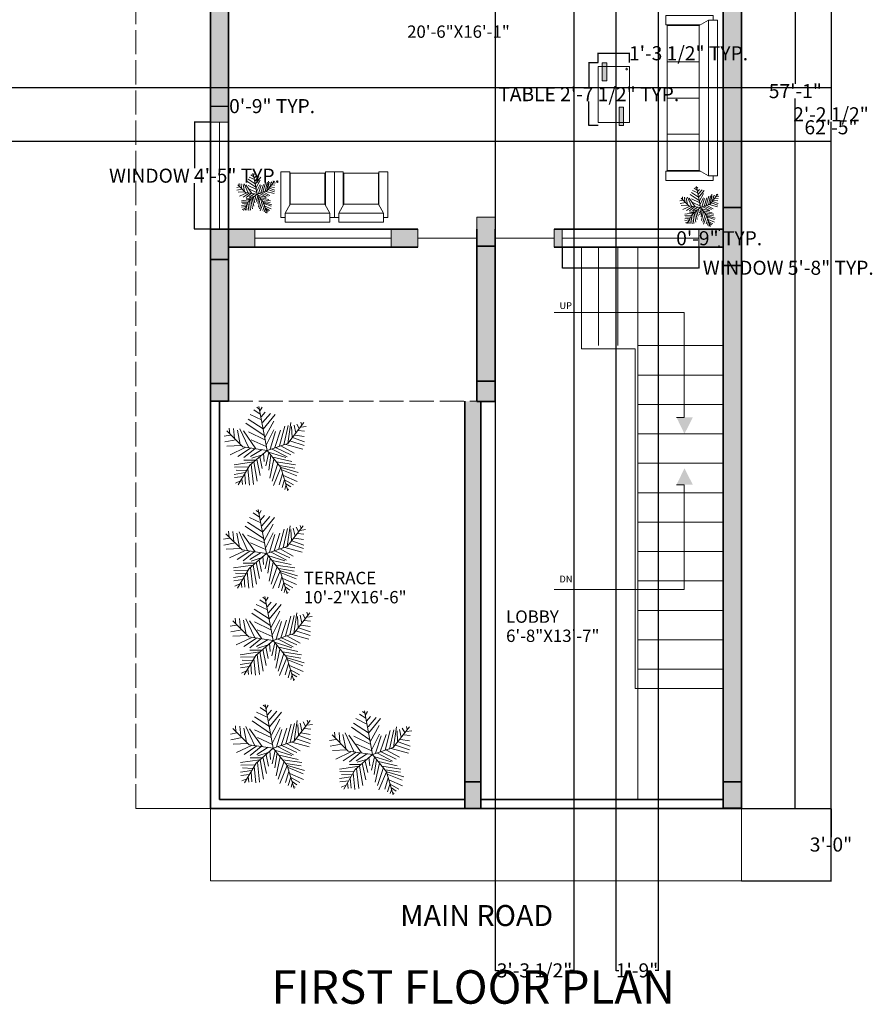
# Model space of a CAD drawing. Units: inches. Extents: x -17 to 892, y -721 to 172.
# Tile 7 of 11: x 438 to 862, y -721 to -231. Entities that reach past the tile are written whole.
import ezdxf

# ---------------------------------------------------------------- set-up
doc = ezdxf.new("R2010")
doc.units = ezdxf.units.IN
doc.header["$MEASUREMENT"] = 0
doc.linetypes.add('ACAD_ISO02W100', pattern=[15, 12, -3])
doc.layers.get('0').update_dxf_attribs({"color": 14})
for name, color, linetype, lineweight in [('A-ANNO-DIMS', 2, 'Continuous', 18), ('A-ANNO-SYMB', 7, 'Continuous', 18), ('A-ANNO-TEXT', 7, 'Continuous', 18), ('A-ANNO-TITL', 7, 'Continuous', 35), ('A-AREA-IDEN', 7, 'Continuous', 18), ('A-COLS', 252, 'Continuous', 35), ('A-FLOR-OVHD', 252, 'ACAD_ISO02W100', 18), ('A-FLOR-STRS', 8, 'Continuous', 18), ('A-WALL-PATT', 14, 'Continuous', 13), ('C-PROP', 8, 'ACAD_ISO02W100', 18), ('C-ROAD', 8, 'Continuous', 18), ('doors', 4, 'Continuous', 18), ('furniture', 252, 'Continuous', 18), ('lawn', 102, 'Continuous', 13), ('walls', 252, 'Continuous', 35), ('windows', 161, 'Continuous', 18)]:
    doc.layers.add(name, color=color, linetype=linetype, lineweight=lineweight)
doc.layers.add('A-COLS-PATT', color=254, linetype='Continuous', lineweight=13, true_color=0xd7ebd2)
doc.styles.get("Standard").update_dxf_attribs({"font": 'arial.ttf'})
doc.dimstyles.get("Standard").update_dxf_attribs({"dimtxt": 7, "dimasz": 0.18, "dimexe": 0.18, "dimexo": 0.0625, "dimgap": 0.09, "dimtad": 0, "dimtih": 1, "dimtoh": 1, "dimzin": 0, "dimdsep": 46, "dimlunit": 3, "dimtxsty": 'Standard', "dimcen": 0.09, "dimadec": 0, "dimazin": 0, "dimtfac": 1, "dimtofl": 0, "dimtmove": 0, "dimatfit": 3, "dimfxl": 1, "dimtolj": 1, "dimtzin": 0, "dimarcsym": 0})

# ---------------------------------------------------------------- blocks, each defined once
blk = doc.blocks.new('FABRIC SOFA 4S')
at = {"layer": 'furniture'}
for p, q in [((3, 54), (34, 54)), ((3, 51), (3, 54)), ((34, 48), (34, 54)), ((0, -51), (0, 51)), ((6, 51), (0, 51)), ((6, -51), (6, 51)), ((12, 47.63), (6, 51)), ((11.14, 48), (34, 48)), ((33, 23.81), (12, 23.81)), ((33, 0), (12, 0)), ((33, -23.81), (12, -23.81)), ((6, -51), (0, -51)), ((3, -54), (3, -51)), ((6, -51), (12, -47.63)), ((11.54, -48), (34, -48)), ((34, -48), (34, -54)), ((3, -54), (34, -54))]:
    blk.add_line(p, q, dxfattribs=at)
blk.add_lwpolyline([(12, -47.63), (12, 47.63), (33, 47.63), (33, -47.63)], close=True, dxfattribs=at)
blk = doc.blocks.new('FABRIC SOFA 1S')
at = {"layer": 'furniture'}
for p, q in [((0, -15.12), (0, 15.12)), ((6, 15.12), (0, 15.12)), ((3, 18.12), (34, 18.12)), ((3, 15.12), (3, 18.12)), ((6, -15.12), (6, 15.12)), ((12, 11.75), (6, 15.12)), ((34, 12.12), (34, 18.12)), ((11.33, 12.12), (34, 12.12)), ((6, -15.12), (12, -11.75)), ((11.33, -12.12), (34, -12.12)), ((34, -12.12), (34, -18.12)), ((6, -15.12), (0, -15.12)), ((3, -18.12), (3, -15.12)), ((3, -18.12), (34, -18.12))]:
    blk.add_line(p, q, dxfattribs=at)
blk.add_lwpolyline([(12, -11.75), (12, 11.75), (33, 11.75), (33, -11.75)], close=True, dxfattribs=at)
blk = doc.blocks.new('*U14')
for p, q in [((-8.737, 47.138), (-17.069, 52.711)), ((-10.186, 53.64), (-13.084, 55.962)), ((0, 0), (-10.5, 57)), ((-9.099, 51.782), (-6.563, 55.962)), ((-5.114, 28.097), (-24.676, 40.636)), ((-7.288, 39.707), (-21.778, 46.673)), ((-7.65, 43.423), (-2.578, 49.46)), ((-5.839, 35.992), (4.667, 48.067)), ((-5.114, 27.632), (10.463, 46.673)), ((-48.585, 21.131), (-49.309, 29.026)), ((-43.513, 28.561), (-42.427, 15.558)), ((-38.442, 26.239), (-34.819, 7.663)), ((-35.544, 28.097), (-24.314, 3.947)), ((-3.665, 19.273), (-27.574, 35.527)), ((-2.941, 16.486), (8.652, 37.85)), ((-1.129, 6.734), (9.014, 26.704)), ((10.101, 3.483), (17.708, 26.239)), ((16.259, 5.805), (23.142, 31.348)), ((22.055, 7.198), (27.489, 32.277)), ((27, 9), (48, 36)), ((27.127, 9.056), (31.112, 35.992)), ((31.836, 30.883), (32.561, 16.486)), ((35.096, 32.741), (37.27, 22.524)), ((38.719, 34.134), (41.979, 28.561)), ((40.53, 25.775), (48.862, 24.846)), ((43.791, 29.954), (51.036, 30.883)), ((44.153, 36.456), (45.239, 32.741)), ((-47.498, 19.737), (-55.83, 18.344)), ((-40.615, 13.7), (-55.105, 10.913)), ((-31.5, 4.5), (-52.5, 25.5)), ((-14.533, 2.09), (-30.834, 25.31)), ((-24.314, 23.917), (-2.941, 13.7)), ((-20.691, 13.7), (-1.129, 4.876)), ((3.942, 1.625), (11.187, 24.381)), ((33.285, 16.486), (48.862, 10.913)), ((36.183, 19.737), (48.137, 17.88)), ((-33.37, 6.269), (-52.207, 5.34)), ((-28.299, 3.483), (-47.86, -5.805)), ((-21.416, 3.018), (-38.079, -8.128)), ((0, 0), (-31.5, 4.5)), ((-15.982, 2.09), (-30.11, -9.521)), ((0, 0), (-22.5, -19.5)), ((-6.563, 1.161), (-21.416, -8.128)), ((0, 0), (27, 9)), ((0, 0), (18, -22.5)), ((6.478, 1.625), (26.04, -8.592)), ((11.187, 3.483), (30.749, -5.805)), ((18.07, 5.805), (35.096, -3.483)), ((24.229, 7.663), (46.688, 1.625)), ((29.662, 12.307), (48.137, 6.269)), ((-15.257, -12.772), (-30.11, -12.772)), ((-6.563, -5.805), (-19.967, -9.985)), ((-13.446, -11.378), (-8.737, -32.741)), ((-9.461, -8.592), (-6.201, -23.453)), ((-4.752, -3.483), (-3.665, -14.629)), ((2.493, -3.019), (-1.491, -20.202)), ((1.769, -2.555), (24.229, -9.521)), ((5.029, -6.27), (2.131, -25.775)), ((9.014, -11.378), (3.58, -35.992)), ((7.565, -9.056), (32.198, -14.629)), ((-17.431, -15.094), (-42.789, -18.809)), ((-24.314, -21.596), (-42.427, -22.06)), ((-22.5, -19.5), (-37.5, -45)), ((-25.038, -23.918), (-22.865, -45.281)), ((-20.691, -18.345), (-17.793, -44.352)), ((-17.069, -15.094), (-12.721, -40.172)), ((14.085, -16.951), (6.478, -40.172)), ((18.07, -22.524), (8.289, -45.745)), ((12.274, -15.094), (36.907, -18.809)), ((16.259, -19.738), (36.183, -22.989)), ((18, -22.5), (27, -52.5)), ((18.433, -22.524), (40.53, -29.026)), ((19.157, -25.311), (38.719, -33.206)), ((-28.299, -29.026), (-42.789, -31.348)), ((-30.834, -34.135), (-42.427, -35.528)), ((-26.849, -26.24), (-40.253, -25.775)), ((-32.646, -36.921), (-31.921, -44.352)), ((-29.023, -30.884), (-27.936, -43.887)), ((20.244, -30.419), (15.897, -44.816)), ((22.78, -37.85), (19.519, -48.532)), ((21.331, -32.741), (39.081, -40.636)), ((22.78, -38.314), (34.372, -44.816)), ((-34.457, -39.708), (-40.978, -42.494)), ((24.591, -45.745), (23.142, -50.854)), ((24.591, -43.423), (30.749, -47.603)), ((26.764, -49.925), (28.213, -50.854))]:
    blk.add_line(p, q)
blk = doc.blocks.new('*D17')
at = {"layer": 'A-ANNO-DIMS', "color": 0, "lineweight": -2, "transparency": 16777216}
for p, q in [((822.86, 89.9), (823.61, 89.9)), ((823.43, 89.72), (823.43, -263.08)), ((823.43, -623.21), (823.43, -270.41)), ((822.86, -623.39), (823.61, -623.39))]:
    blk.add_line(p, q, dxfattribs=at)
at = {"layer": 'A-ANNO-DIMS', "color": 0, "lineweight": 100, "transparency": 16777216}
for points in [[(823.4, 89.72), (823.46, 89.72), (823.43, 89.9)], [(823.4, -623.21), (823.46, -623.21), (823.43, -623.39)]]:
    blk.add_solid(points, dxfattribs=at)
at = {"layer": 'Defpoints', "color": 0, "lineweight": 100, "transparency": 16777216}
for p in [(822.8, 89.9), (822.8, -623.39), (823.43, -623.39)]:
    blk.add_point(p, dxfattribs=at)
at = {"layer": 'A-ANNO-DIMS', "color": 0, "transparency": 16777216, "insert": (823.43, -266.74), "char_height": 7, "attachment_point": 5}
blk.add_mtext('\\A1;57\'-1"', dxfattribs=at)
blk = doc.blocks.new('WIN-68-INSET')
for p, q in [((0, 9), (0, 0)), ((0, 9), (0, 4.5)), ((67.89, 0), (67.89, 9)), ((0, 4.5), (67.89, 4.5))]:
    blk.add_line(p, q)
blk = doc.blocks.new('WIN-53-INSET')
for p, q in [((0, 53.21), (9, 53.21)), ((0, 53.21), (4.5, 53.21)), ((4.5, 53.21), (4.5, 0)), ((9, 0), (0, 0))]:
    blk.add_line(p, q)
blk = doc.blocks.new('TABLE-COCKTAIL')
h = blk.add_hatch(color=256)
h.dxf.hatch_style = 1
h.paths.add_polyline_path([(4.23, 29.31), (2.04, 29.31), (2.04, 22.19), (4.23, 22.19)])
h.paths.add_polyline_path([(4.23, 31.28), (2.04, 31.28), (2.04, 29.31), (4.23, 29.31)])
h.paths.add_polyline_path([(12.58, 9.09), (10.39, 9.09), (10.39, 1.62), (12.58, 1.62)])
h.paths.add_polyline_path([(12.58, 1.62), (10.39, 1.62), (10.39, 0), (12.58, 0)])
for p, q in [((2.04, 31.28), (4.23, 31.28)), ((2.04, 22.19), (2.04, 31.28)), ((4.23, 31.28), (4.23, 22.19)), ((0, 29.31), (0, 1.62)), ((15.53, 29.31), (0, 29.31)), ((15.53, 1.62), (15.53, 29.31)), ((4.23, 22.19), (2.04, 22.19)), ((10.39, 9.09), (12.58, 9.09)), ((10.39, 0), (10.39, 9.09)), ((12.58, 9.09), (12.58, 0)), ((0, 1.62), (15.53, 1.62)), ((12.58, 0), (10.39, 0))]:
    blk.add_line(p, q)
blk.add_circle((14.17, 28.1), 0.401)
blk = doc.blocks.new('STAIR-DIRECTION')
h = blk.add_hatch(color=256)
h.dxf.hatch_style = 1
h.paths.add_polyline_path([(64.68, 8.16), (60.81, 8.16), (64.68, 0.16)])
h.paths.add_polyline_path([(68.92, 8.16), (64.68, 8.16), (64.68, 0.16), (64.75, 0)])
for p, q in [((0, 60.33), (64.68, 60.33)), ((64.68, 60.33), (64.68, 8.16)), ((64.68, 8.16), (60.81, 8.16))]:
    blk.add_line(p, q)
blk = doc.blocks.new('*D34')
at = {"layer": 'A-ANNO-DIMS', "color": 0, "lineweight": -2, "transparency": 16777216}
for p, q in [((707.47, -344.45), (707.47, -354.75)), ((775.36, -344.45), (775.36, -354.75)), ((707.65, -354.57), (775.18, -354.57)), ((775.36, -354.57), (775.54, -354.57))]:
    blk.add_line(p, q, dxfattribs=at)
at = {"layer": 'A-ANNO-DIMS', "color": 0, "lineweight": 100, "transparency": 16777216}
for points in [[(707.65, -354.54), (707.65, -354.6), (707.47, -354.57)], [(775.18, -354.54), (775.18, -354.6), (775.36, -354.57)]]:
    blk.add_solid(points, dxfattribs=at)
at = {"layer": 'Defpoints', "color": 0, "lineweight": 100, "transparency": 16777216}
for p in [(707.47, -344.39), (775.36, -344.39), (775.36, -354.57)]:
    blk.add_point(p, dxfattribs=at)
at = {"layer": 'A-ANNO-DIMS', "color": 0, "transparency": 16777216, "insert": (819.92, -354.57), "char_height": 7, "attachment_point": 5}
blk.add_mtext('\\A1;WINDOW 5\'-8" TYP.', dxfattribs=at)
blk = doc.blocks.new('*D35')
at = {"layer": 'A-ANNO-DIMS', "color": 0, "lineweight": -2, "transparency": 16777216}
for p, q in [((775.42, -335.39), (785.73, -335.39)), ((785.55, -335.57), (785.55, -336.23)), ((775.42, -344.39), (785.73, -344.39)), ((785.55, -344.21), (785.55, -343.55))]:
    blk.add_line(p, q, dxfattribs=at)
at = {"layer": 'A-ANNO-DIMS', "color": 0, "lineweight": 100, "transparency": 16777216}
for points in [[(785.52, -335.57), (785.58, -335.57), (785.55, -335.39)], [(785.52, -344.21), (785.58, -344.21), (785.55, -344.39)]]:
    blk.add_solid(points, dxfattribs=at)
at = {"layer": 'Defpoints', "color": 0, "lineweight": 100, "transparency": 16777216}
for p in [(775.36, -335.39), (785.55, -335.39), (775.36, -344.39)]:
    blk.add_point(p, dxfattribs=at)
at = {"layer": 'A-ANNO-DIMS', "color": 0, "transparency": 16777216, "insert": (785.55, -339.89), "char_height": 7, "attachment_point": 5}
blk.add_mtext('\\A1;0\'-9" TYP.', dxfattribs=at)
blk = doc.blocks.new('*D42')
at = {"layer": 'A-ANNO-DIMS', "color": 0, "lineweight": -2, "transparency": 16777216}
for p, q in [((725.31, -252.61), (720.5, -252.61)), ((720.68, -252.79), (720.68, -264.54)), ((720.68, -283.71), (720.68, -271.96)), ((725.31, -283.89), (720.5, -283.89))]:
    blk.add_line(p, q, dxfattribs=at)
at = {"layer": 'A-ANNO-DIMS', "color": 0, "lineweight": 100, "transparency": 16777216}
for points in [[(720.65, -252.79), (720.71, -252.79), (720.68, -252.61)], [(720.65, -283.71), (720.71, -283.71), (720.68, -283.89)]]:
    blk.add_solid(points, dxfattribs=at)
at = {"layer": 'Defpoints', "color": 0, "lineweight": 100, "transparency": 16777216}
for p in [(720.68, -252.61), (725.37, -252.61), (725.37, -283.89)]:
    blk.add_point(p, dxfattribs=at)
at = {"layer": 'A-ANNO-DIMS', "color": 0, "transparency": 16777216, "insert": (720.68, -268.25), "char_height": 7, "attachment_point": 5}
blk.add_mtext('\\A1;TABLE 2\'-7 1/2" TYP.', dxfattribs=at)
blk = doc.blocks.new('*D43')
at = {"layer": 'A-ANNO-DIMS', "color": 0, "lineweight": -2, "transparency": 16777216}
for p, q in [((725.37, -252.55), (725.37, -247.74)), ((725.55, -247.92), (740.71, -247.92)), ((740.89, -252.55), (740.89, -247.74)), ((740.89, -247.92), (741.07, -247.92))]:
    blk.add_line(p, q, dxfattribs=at)
at = {"layer": 'A-ANNO-DIMS', "color": 0, "lineweight": 100, "transparency": 16777216}
for points in [[(725.55, -247.89), (725.55, -247.95), (725.37, -247.92)], [(740.71, -247.89), (740.71, -247.95), (740.89, -247.92)]]:
    blk.add_solid(points, dxfattribs=at)
at = {"layer": 'Defpoints', "color": 0, "lineweight": 100, "transparency": 16777216}
for p in [(740.89, -247.92), (725.37, -252.61), (740.89, -252.61)]:
    blk.add_point(p, dxfattribs=at)
at = {"layer": 'A-ANNO-DIMS', "color": 0, "transparency": 16777216, "insert": (770.32, -247.92), "char_height": 7, "attachment_point": 5}
blk.add_mtext('\\A1;1\'-3 1/2" TYP.', dxfattribs=at)
blk = doc.blocks.new('*D46')
at = {"layer": 'A-ANNO-DIMS', "color": 0, "lineweight": -2, "transparency": 16777216}
for p, q in [((532.51, -282.18), (524.41, -282.18)), ((524.59, -282.36), (524.59, -305.07)), ((524.59, -335.21), (524.59, -312.5)), ((532.51, -335.39), (524.41, -335.39))]:
    blk.add_line(p, q, dxfattribs=at)
at = {"layer": 'A-ANNO-DIMS', "color": 0, "lineweight": 100, "transparency": 16777216}
for points in [[(524.56, -282.36), (524.62, -282.36), (524.59, -282.18)], [(524.56, -335.21), (524.62, -335.21), (524.59, -335.39)]]:
    blk.add_solid(points, dxfattribs=at)
at = {"layer": 'Defpoints', "color": 0, "lineweight": 100, "transparency": 16777216}
for p in [(524.59, -282.18), (532.58, -282.18), (532.58, -335.39)]:
    blk.add_point(p, dxfattribs=at)
at = {"layer": 'A-ANNO-DIMS', "color": 0, "transparency": 16777216, "insert": (524.59, -308.79), "char_height": 7, "attachment_point": 5}
blk.add_mtext('\\A1;WINDOW 4\'-5" TYP.', dxfattribs=at)
blk = doc.blocks.new('*D47')
at = {"layer": 'A-ANNO-DIMS', "color": 0, "lineweight": -2, "transparency": 16777216}
for p, q in [((532.58, -282.12), (532.58, -274.02)), ((541.58, -282.12), (541.58, -274.02)), ((532.76, -274.2), (541.4, -274.2)), ((541.58, -274.2), (541.76, -274.2))]:
    blk.add_line(p, q, dxfattribs=at)
at = {"layer": 'A-ANNO-DIMS', "color": 0, "lineweight": 100, "transparency": 16777216}
for points in [[(532.76, -274.17), (532.76, -274.23), (532.58, -274.2)], [(541.4, -274.17), (541.4, -274.23), (541.58, -274.2)]]:
    blk.add_solid(points, dxfattribs=at)
at = {"layer": 'Defpoints', "color": 0, "lineweight": 100, "transparency": 16777216}
for p in [(541.58, -274.2), (532.58, -282.18), (541.58, -282.18)]:
    blk.add_point(p, dxfattribs=at)
at = {"layer": 'A-ANNO-DIMS', "color": 0, "transparency": 16777216, "insert": (563.18, -274.2), "char_height": 7, "attachment_point": 5}
blk.add_mtext('\\A1;0\'-9" TYP.', dxfattribs=at)
blk = doc.blocks.new('*D59')
at = {"layer": 'A-ANNO-DIMS', "color": 0, "lineweight": -2, "transparency": 16777216}
for p, q in [((796.64, 89.9), (841.36, 89.9)), ((841.18, 89.72), (841.18, -281.05)), ((841.18, -659.16), (841.18, -288.38)), ((796.64, -659.34), (841.36, -659.34))]:
    blk.add_line(p, q, dxfattribs=at)
at = {"layer": 'A-ANNO-DIMS', "color": 0, "lineweight": 100, "transparency": 16777216}
for points in [[(841.15, 89.72), (841.21, 89.72), (841.18, 89.9)], [(841.15, -659.16), (841.21, -659.16), (841.18, -659.34)]]:
    blk.add_solid(points, dxfattribs=at)
at = {"layer": 'Defpoints', "color": 0, "lineweight": 100, "transparency": 16777216}
for p in [(796.58, 89.9), (841.18, 89.9), (796.58, -659.34)]:
    blk.add_point(p, dxfattribs=at)
at = {"layer": 'A-ANNO-DIMS', "color": 0, "transparency": 16777216, "insert": (841.18, -284.72), "char_height": 7, "attachment_point": 5}
blk.add_mtext('\\A1;62\'-5"', dxfattribs=at)
blk = doc.blocks.new('*D61')
at = {"layer": 'A-ANNO-DIMS', "color": 0, "lineweight": -2, "transparency": 16777216}
for p, q in [((170.99, -264.92), (841.36, -264.92)), ((841.18, -265.1), (841.18, -274.56)), ((841.18, -291.45), (841.18, -281.98)), ((170.99, -291.63), (841.36, -291.63))]:
    blk.add_line(p, q, dxfattribs=at)
at = {"layer": 'A-ANNO-DIMS', "color": 0, "lineweight": 100, "transparency": 16777216}
for points in [[(841.15, -265.1), (841.21, -265.1), (841.18, -264.92)], [(841.15, -291.45), (841.21, -291.45), (841.18, -291.63)]]:
    blk.add_solid(points, dxfattribs=at)
at = {"layer": 'Defpoints', "color": 0, "lineweight": 100, "transparency": 16777216}
for p in [(170.93, -264.92), (170.93, -291.63), (841.18, -291.63)]:
    blk.add_point(p, dxfattribs=at)
at = {"layer": 'A-ANNO-DIMS', "color": 0, "transparency": 16777216, "insert": (841.18, -278.27), "char_height": 7, "attachment_point": 5}
blk.add_mtext('\\A1;2\'-2 1/2"', dxfattribs=at)
blk = doc.blocks.new('*D62')
at = {"layer": 'A-ANNO-DIMS', "color": 0, "lineweight": -2, "transparency": 16777216}
for p, q in [((674.08, -154.45), (674.08, -704.12)), ((713.34, -154.45), (713.34, -704.12)), ((674.26, -703.94), (676.16, -703.94)), ((713.16, -703.94), (711.26, -703.94))]:
    blk.add_line(p, q, dxfattribs=at)
at = {"layer": 'A-ANNO-DIMS', "color": 0, "lineweight": 100, "transparency": 16777216}
for points in [[(674.26, -703.91), (674.26, -703.97), (674.08, -703.94)], [(713.16, -703.91), (713.16, -703.97), (713.34, -703.94)]]:
    blk.add_solid(points, dxfattribs=at)
at = {"layer": 'Defpoints', "color": 0, "lineweight": 100, "transparency": 16777216}
for p in [(674.08, -154.39), (713.34, -154.39), (713.34, -703.94)]:
    blk.add_point(p, dxfattribs=at)
at = {"layer": 'A-ANNO-DIMS', "color": 0, "transparency": 16777216, "insert": (693.71, -703.94), "char_height": 7, "attachment_point": 5}
blk.add_mtext('\\A1;3\'-3 1/2"', dxfattribs=at)
blk = doc.blocks.new('*D65')
at = {"layer": 'A-ANNO-DIMS', "color": 0, "lineweight": -2, "transparency": 16777216}
for p, q in [((796.64, -623.39), (841.36, -623.39)), ((841.18, -623.57), (841.18, -637.7)), ((841.18, -659.16), (841.18, -645.03)), ((796.64, -659.34), (841.36, -659.34))]:
    blk.add_line(p, q, dxfattribs=at)
at = {"layer": 'A-ANNO-DIMS', "color": 0, "lineweight": 100, "transparency": 16777216}
for points in [[(841.15, -623.57), (841.21, -623.57), (841.18, -623.39)], [(841.15, -659.16), (841.21, -659.16), (841.18, -659.34)]]:
    blk.add_solid(points, dxfattribs=at)
at = {"layer": 'Defpoints', "color": 0, "lineweight": 100, "transparency": 16777216}
for p in [(796.58, -623.39), (796.58, -659.34), (841.18, -659.34)]:
    blk.add_point(p, dxfattribs=at)
at = {"layer": 'A-ANNO-DIMS', "color": 0, "transparency": 16777216, "insert": (841.18, -641.36), "char_height": 7, "attachment_point": 5}
blk.add_mtext('\\A1;3\'-0"', dxfattribs=at)
blk = doc.blocks.new('*D67')
at = {"layer": 'A-ANNO-DIMS', "color": 0, "lineweight": -2, "transparency": 16777216}
for p, q in [((734.21, 32.4), (734.21, -704.12)), ((755.21, 32.4), (755.21, -704.12)), ((734.39, -703.94), (735.64, -703.94)), ((755.03, -703.94), (753.77, -703.94))]:
    blk.add_line(p, q, dxfattribs=at)
at = {"layer": 'A-ANNO-DIMS', "color": 0, "lineweight": 100, "transparency": 16777216}
for points in [[(734.39, -703.91), (734.39, -703.97), (734.21, -703.94)], [(755.03, -703.91), (755.03, -703.97), (755.21, -703.94)]]:
    blk.add_solid(points, dxfattribs=at)
at = {"layer": 'Defpoints', "color": 0, "lineweight": 100, "transparency": 16777216}
for p in [(734.21, 32.46), (755.21, 32.46), (755.21, -703.94)]:
    blk.add_point(p, dxfattribs=at)
at = {"layer": 'A-ANNO-DIMS', "color": 0, "transparency": 16777216, "insert": (744.71, -703.94), "char_height": 7, "attachment_point": 5}
blk.add_mtext('\\A1;1\'-9"', dxfattribs=at)

msp = doc.modelspace()

# ---------------------------------------------------------------- hatches: boundary and pattern name
at = {"layer": 'A-COLS-PATT'}
h = msp.add_hatch(color=256, dxfattribs=at)
h.dxf.hatch_style = 1
h.paths.add_polyline_path([(796.576, 61.611), (787.576, 61.611), (787.576, 43.692), (796.576, 43.692)])
h.paths.add_polyline_path([(796.576, -140.181), (787.576, -140.181), (787.576, -157.529), (796.576, -157.529)])
h.paths.add_polyline_path([(674.076, -107.889), (665.076, -107.889), (665.076, -116.615), (674.076, -116.615)])
h.paths.add_polyline_path([(537.076, -107.889), (532.576, -107.889), (532.576, -116.615), (537.076, -116.615)])
h.paths.add_polyline_path([(541.576, -207.597), (532.576, -207.597), (532.576, -223.04), (541.576, -223.04)])
h.paths.add_polyline_path([(541.576, -335.389), (532.576, -335.389), (532.576, -350.421), (541.576, -350.421)])
h.paths.add_polyline_path([(541.576, -412.049), (532.576, -412.049), (532.576, -420.971), (541.576, -420.971)])
h.paths.add_polyline_path([(674.076, -410.999), (665.076, -410.999), (665.076, -421.003), (674.076, -421.003)])
h.paths.add_polyline_path([(674.076, -329.432), (665.076, -329.432), (665.076, -335.389), (665.076, -343.822), (674.076, -343.822), (674.076, -335.389)])
h.paths.add_polyline_path([(667.076, -610.134), (659.076, -610.134), (659.076, -618.889), (659.101, -623.389), (667.076, -623.389)])
h.paths.add_polyline_path([(796.576, -610.134), (787.576, -610.134), (787.576, -614.389), (787.576, -623.342), (796.576, -623.342)])
h.paths.add_polyline_path([(796.576, -324.682), (787.576, -324.682), (787.576, -353.487), (796.576, -353.487)])
at = {"layer": 'A-WALL-PATT'}
h = msp.add_hatch(color=256, dxfattribs=at)
h.dxf.hatch_style = 1
h.paths.add_polyline_path([(669.576, 4.611), (787.576, 4.611), (787.576, 9.111), (669.576, 9.111), (669.576, 53.097), (665.076, 53.097), (665.076, -107.889), (669.576, -107.889)])
h.paths.add_polyline_path([(674.076, -116.615), (665.076, -116.615), (665.076, -154.389), (674.076, -154.389)])
h.paths.add_polyline_path([(787.576, -145.389), (713.344, -145.389), (713.344, -154.389), (787.576, -154.389)])
h.paths.add_polyline_path([(632.137, -145.389), (622.476, -145.389), (622.476, -154.389), (632.137, -154.389)])
h.paths.add_polyline_path([(554.583, -145.389), (537.076, -145.389), (537.076, -154.389), (554.583, -154.389)])
h.paths.add_polyline_path([(537.076, -145.389), (532.576, -145.389), (532.576, -154.389), (537.076, -154.389)])
h.paths.add_polyline_path([(537.076, -116.615), (532.576, -116.615), (532.576, -145.389), (537.076, -145.389)])
h.paths.add_polyline_path([(796.576, 43.692), (787.576, 43.692), (787.576, -140.181), (796.576, -140.181)])
h.paths.add_polyline_path([(541.576, -223.04), (532.576, -223.04), (532.576, -282.182), (537.076, -282.182), (541.576, -282.182)])
h.paths.add_polyline_path([(796.576, -157.529), (787.576, -157.529), (787.576, -324.682), (796.576, -324.682)])
h.paths.add_polyline_path([(554.583, -335.389), (541.576, -335.389), (541.576, -344.389), (554.583, -344.389)])
h.paths.add_polyline_path([(635.731, -335.389), (622.476, -335.389), (622.476, -344.389), (635.731, -344.389)])
h.paths.add_polyline_path([(541.576, -350.421), (532.576, -350.421), (532.576, -412.049), (541.576, -412.049)])
h.paths.add_polyline_path([(674.076, -343.822), (665.076, -343.822), (665.076, -410.999), (674.076, -410.999)])
h.paths.add_polyline_path([(667.076, -421.003), (665.076, -421.003), (659.076, -421.002), (659.076, -610.134), (667.076, -610.134)])
h.paths.add_polyline_path([(796.576, -353.487), (787.576, -353.487), (787.576, -610.134), (796.576, -610.134)])
h.paths.add_polyline_path([(787.576, -335.389), (775.362, -335.389), (775.362, -344.389), (787.576, -344.389)])
h.paths.add_polyline_path([(707.469, -335.389), (703.501, -335.389), (703.501, -344.389), (707.469, -344.389)])
h.paths.add_polyline_path([(695.494, 61.611), (676.541, 61.611), (676.541, 57.111), (695.494, 57.111)])
h.paths.add_polyline_path([(729.183, 61.611), (724.076, 61.611), (711.12, 61.611), (711.12, 57.111), (729.183, 57.111)])
h.paths.add_polyline_path([(787.576, 61.611), (735.904, 61.611), (735.904, 57.111), (787.576, 57.111)])

# ---------------------------------------------------------------- linework, layer by layer
at = {"layer": 'A-COLS'}
for p, q in [((787.576, -324.682), (796.576, -324.682)), ((665.076, -343.822), (674.076, -343.822)), ((532.576, -350.421), (541.576, -350.421)), ((787.576, -353.487), (796.576, -353.487)), ((665.076, -410.999), (674.076, -410.999)), ((532.576, -412.049), (541.576, -412.049)), ((532.576, -420.971), (541.576, -420.971)), ((665.076, -421.003), (674.076, -421.003)), ((659.076, -610.134), (667.076, -610.134)), ((667.076, -610.134), (667.076, -623.389)), ((787.576, -610.134), (796.576, -610.134)), ((787.576, -623.342), (787.576, -614.389)), ((659.101, -623.389), (659.076, -618.889)), ((667.076, -623.389), (659.101, -623.389)), ((787.576, -623.342), (796.576, -623.342))]:
    msp.add_line(p, q, dxfattribs=at)
at = {"layer": 'A-FLOR-OVHD'}
for p, q in [((665.076, -335.389), (665.076, -329.432)), ((665.076, -329.432), (674.076, -329.432)), ((674.076, -329.432), (674.076, -335.389)), ((635.731, -335.389), (635.731, -344.389)), ((703.501, -335.389), (703.501, -344.389)), ((541.576, -420.971), (665.076, -420.971))]:
    msp.add_line(p, q, dxfattribs=at)
at = {"layer": 'A-FLOR-STRS'}
for p, q in [((717.124, -344.389), (717.124, -394.824)), ((725.526, -344.389), (725.526, -393.266)), ((735.202, -344.389), (735.202, -393.266)), ((745.042, -344.389), (745.042, -393.266)), ((717.124, -394.824), (743.848, -394.824)), ((743.848, -394.824), (743.848, -563.768)), ((745.042, -393.266), (745.042, -618.889)), ((745.042, -393.266), (787.576, -393.266)), ((745.042, -407.895), (787.576, -407.895)), ((745.042, -422.524), (787.576, -422.524)), ((745.042, -437.153), (787.576, -437.153)), ((745.042, -451.781), (787.576, -451.781)), ((745.042, -466.41), (787.576, -466.41)), ((745.042, -481.039), (787.576, -481.039)), ((745.042, -495.668), (787.576, -495.668)), ((745.042, -510.297), (787.576, -510.297)), ((745.042, -524.926), (787.576, -524.926)), ((745.042, -539.555), (787.576, -539.555)), ((745.042, -554.184), (787.576, -554.184)), ((743.848, -563.768), (787.576, -563.768))]:
    msp.add_line(p, q, dxfattribs=at)
at = {"layer": 'C-PROP'}
msp.add_line((495.384, -623.389), (495.384, 61.611), dxfattribs=at)
at = {"layer": 'C-ROAD'}
for p, q in [((532.576, -623.389), (495.384, -623.389)), ((532.576, -623.389), (532.576, -659.336)), ((796.576, -659.336), (796.576, -623.389)), ((532.576, -659.336), (796.576, -659.336))]:
    msp.add_line(p, q, dxfattribs=at)
at = {"layer": 'doors'}
for p, q in [((635.731, -339.889), (665.076, -339.889)), ((703.501, -339.889), (674.076, -339.889))]:
    msp.add_line(p, q, dxfattribs=at)
at = {"layer": 'walls'}
for p, q in [((532.576, -623.389), (532.576, 61.611)), ((787.576, 61.611), (787.576, -614.389)), ((796.576, 61.611), (796.576, -623.389)), ((541.576, -420.971), (541.576, -154.389)), ((532.576, -335.389), (635.731, -335.389)), ((665.076, -420.971), (665.076, -335.389)), ((674.076, -421.003), (674.076, -335.389)), ((703.501, -335.389), (787.576, -335.389)), ((541.576, -344.389), (635.731, -344.389)), ((703.501, -344.389), (787.576, -344.389)), ((537.076, -618.889), (537.076, -420.971)), ((537.076, -618.889), (537.076, -420.971)), ((659.076, -618.889), (659.076, -420.971)), ((667.076, -618.889), (667.076, -420.971)), ((659.076, -618.889), (537.076, -618.889)), ((787.576, -618.889), (667.076, -618.889)), ((796.576, -623.389), (532.576, -623.389)), ((668.576, -623.389), (670.658, -623.389)), ((796.576, -623.389), (711.765, -623.389))]:
    msp.add_line(p, q, dxfattribs=at)

# ---------------------------------------------------------------- block references
at = {"layer": 'A-ANNO-SYMB'}
msp.add_blockref('STAIR-DIRECTION', (703.533, -437.153), dxfattribs=at)
at = {"layer": 'A-ANNO-SYMB', "extrusion": (0, 0, -1), "zscale": -1, "rotation": 180}
msp.add_blockref('STAIR-DIRECTION', (-703.533, -454.294), dxfattribs=at)
at = {"layer": 'furniture'}
for name, p, xscale, yscale, zscale, rotation in [('FABRIC SOFA 4S', (784.756, -270.167), 0.7583822975527559, 0.7583822975527559, 0.7583822975527559, 180), ('FABRIC SOFA 1S', (580.841, -331.822), 0.7339463821036302, 0.7339463821036302, 0.7339463821036302, 90.00000000000087), ('FABRIC SOFA 1S', (607.446, -331.822), 0.7339463821036302, 0.7339463821036302, 0.7339463821036302, 90)]:
    msp.add_blockref(name, p, dxfattribs=dict(at, xscale=xscale, yscale=yscale, zscale=zscale, rotation=rotation))
msp.add_blockref('TABLE-COCKTAIL', (725.369, -283.892), dxfattribs=at)
at = {"layer": 'lawn'}
for p, xscale, yscale, zscale in [((555.692, -317.964), 0.1813548619598531, 0.1813548619598531, 0.1813548619598531), ((776.184, -324.586), 0.1813548619598531, 0.1813548619598531, 0.1813548619598531), ((560.668, -445.352), 0.3823150569682844, 0.3823150569682844, 0.3823150569682844), ((560.324, -496.604), 0.3823150569682844, 0.3823150569682844, 0.3823150569682844), ((563.653, -539.838), 0.3823150569682844, 0.3823150569682844, 0.3823150569682844), ((563.789, -593.446), 0.3823150569682844, 0.3823150569682844, 0.3823150569682844), ((613.14, -596.612), 0.3823150569682844, 0.3823150569682844, 0.3823150569682844)]:
    msp.add_blockref('*U14', p, dxfattribs=dict(at, xscale=xscale, yscale=yscale, zscale=zscale))
at = {"layer": 'windows'}
for name, p in [('WIN-53-INSET', (532.576, -335.389)), ('WIN-68-INSET', (554.583, -344.389)), ('WIN-68-INSET', (707.468, -344.389))]:
    msp.add_blockref(name, p, dxfattribs=at)

# ---------------------------------------------------------------- texts
at = {"layer": 'A-ANNO-SYMB'}
for s, p in [('UP', (706.111, -375.084)), ('DN', (706.111, -511.034))]:
    msp.add_text(s, height=3.3722, dxfattribs=at).set_placement(p)
at = {"layer": 'A-ANNO-TEXT'}
msp.add_text('MAIN ROAD', height=10.4498, dxfattribs=at).set_placement((626.917, -681.884))
at = {"layer": 'A-ANNO-TITL'}
msp.add_text('FIRST FLOOR PLAN', height=16.63981, dxfattribs=at).set_placement((562.858, -720.506))
at = {"layer": 'A-AREA-IDEN'}
for s, p in [('20\'-6"X16\'-1"', (630.34, -240.237)), ('TERRACE', (578.991, -511.899)), ('10\'-2"X16\'-6"', (578.991, -521.434)), ('LOBBY', (679.563, -531.1)), ('6\'-8"X13\'-7"', (679.563, -540.634))]:
    msp.add_text(s, height=6.1361, dxfattribs=at).set_placement(p)

# ---------------------------------------------------------------- dimensions: what is measured, and where the dimension line sits
at = {"layer": 'A-ANNO-DIMS'}
for base, p1, p2, picture, middle in [((841.176, 89.902), (796.576, -659.336), (796.576, 89.902), '*D59', (841.176, -284.717)), ((841.176, -291.625), (170.932, -264.917), (170.932, -291.625), '*D61', (841.176, -278.271)), ((841.176, -659.336), (796.576, -623.389), (796.576, -659.336), '*D65', (841.176, -641.363))]:
    dim = msp.add_linear_dim(base=base, p1=p1, p2=p2, angle=90, dimstyle='Standard', override={"dimdec": 1, "dimlfac": 1, "dimrnd": 0, "dimzin": 1, "dimdsep": 46, "dimlunit": 4, "dimfrac": 2}, dxfattribs=at)
    dim.commit()
    dim.dimension.update_dxf_attribs({"geometry": picture, "text_midpoint": middle})
for base, p1, p2, text, override, picture, middle in [((823.427, -623.389), (822.802, 89.902), (822.802, -623.389), '57\'-1"', {"dimclrd": 0, "dimclre": 0, "dimclrt": 0}, '*D17', (823.427, -266.744)), ((720.677, -252.615), (725.369, -283.893), (725.369, -252.615), 'TABLE <> TYP.', {"dimdec": 1, "dimlfac": 1, "dimrnd": 0, "dimzin": 1, "dimdsep": 46, "dimlunit": 4, "dimfrac": 2}, '*D42', (720.677, -268.254)), ((524.595, -282.182), (532.576, -335.389), (532.576, -282.182), 'WINDOW <> TYP.', {"dimdec": 1, "dimlfac": 1, "dimrnd": 0, "dimzin": 1, "dimdsep": 46, "dimlunit": 4, "dimfrac": 2}, '*D46', (524.595, -308.785)), ((785.546, -335.389), (775.362, -344.389), (775.362, -335.389), '<> TYP.', {"dimdec": 1, "dimlfac": 1, "dimrnd": 0, "dimzin": 1, "dimdsep": 46, "dimlunit": 4, "dimfrac": 2}, '*D35', (785.546, -339.889))]:
    dim = msp.add_linear_dim(base=base, p1=p1, p2=p2, angle=90, text=text, dimstyle='Standard', override=override, dxfattribs=at)
    dim.commit()
    dim.dimension.update_dxf_attribs({"geometry": picture, "text_midpoint": middle})
for base, p1, p2, picture, middle in [((755.209, -703.936), (734.209, 32.461), (755.209, 32.461), '*D67', (744.709, -703.936)), ((713.344, -703.936), (674.076, -154.389), (713.344, -154.389), '*D62', (693.71, -703.936))]:
    dim = msp.add_linear_dim(base=base, p1=p1, p2=p2, dimstyle='Standard', override={"dimdec": 1, "dimlfac": 1, "dimrnd": 0, "dimzin": 1, "dimdsep": 46, "dimlunit": 4, "dimfrac": 2}, dxfattribs=at)
    dim.commit()
    dim.dimension.update_dxf_attribs({"geometry": picture, "text_midpoint": middle})
for base, p1, p2, text, picture, middle in [((740.894, -247.923), (725.369, -252.615), (740.894, -252.615), '<> TYP.', '*D43', (770.324, -247.923)), ((541.576, -274.2), (532.576, -282.182), (541.576, -282.182), '<> TYP.', '*D47', (563.18, -274.2)), ((775.362, -354.573), (707.469, -344.389), (775.362, -344.389), 'WINDOW <> TYP.', '*D34', (819.922, -354.573))]:
    dim = msp.add_linear_dim(base=base, p1=p1, p2=p2, text=text, dimstyle='Standard', override={"dimdec": 1, "dimlfac": 1, "dimrnd": 0, "dimzin": 1, "dimdsep": 46, "dimlunit": 4, "dimfrac": 2}, dxfattribs=at)
    dim.commit()
    dim.dimension.update_dxf_attribs({"geometry": picture, "text_midpoint": middle})

doc.saveas('drawing.dxf')
